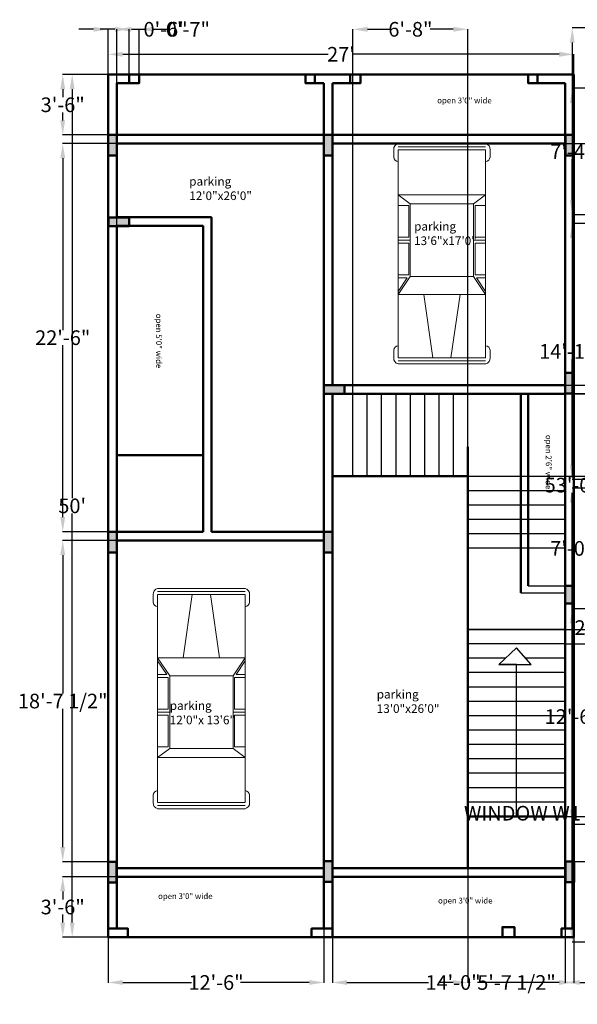
# Model space of a CAD drawing. Units: inches. Extents: x 41 to 5965, y 7 to 3328.
# Tile 1 of 6: x 5054 to 5442, y 1735 to 2420. Entities that reach past the tile are written whole.
import ezdxf

# ---------------------------------------------------------------- set-up
doc = ezdxf.new("R2010")
doc.units = ezdxf.units.IN
doc.header["$MEASUREMENT"] = 0
for name, color, linetype, lineweight in [('A-ANNO-DIMS', 2, 'Continuous', 18), ('A-AREA-IDEN', 3, 'Continuous', 18), ('A-FLOR-STRS', 3, 'Continuous', 25), ('A-FURN', 8, 'Continuous', 18), ('A-WALL', 7, 'Continuous', 50), ('A-WALL-PATT', 8, 'Continuous', 13)]:
    doc.layers.add(name, color=color, linetype=linetype, lineweight=lineweight)
doc.styles.get("Standard").update_dxf_attribs({"font": 'arial.ttf'})
doc.dimstyles.get("Standard").update_dxf_attribs({"dimtxt": 10.18, "dimasz": 10.18, "dimexe": 0.18, "dimexo": 0.0625, "dimgap": 0.09, "dimtad": 0, "dimtih": 1, "dimtoh": 1, "dimdec": 0, "dimzin": 0, "dimdsep": 46, "dimlunit": 3, "dimtxsty": 'Standard', "dimcen": 0.09, "dimadec": 0, "dimazin": 0, "dimtfac": 1, "dimtdec": 0, "dimtofl": 0, "dimtmove": 0, "dimatfit": 3, "dimfxl": 1, "dimtolj": 1, "dimtzin": 0, "dimarcsym": 0})

# ---------------------------------------------------------------- blocks, each defined once
blk = doc.blocks.new('*D1')
at = {"layer": 'A-ANNO-DIMS', "color": 0, "lineweight": -2, "transparency": 16777216}
for p, q in [((5115.3, 2382.15), (5115.3, 2396.38)), ((5125.48, 2396.2), (5268.48, 2396.2)), ((5429.12, 2396.2), (5286.11, 2396.2)), ((5439.3, 2382.15), (5439.3, 2396.38))]:
    blk.add_line(p, q, dxfattribs=at)
at = {"layer": 'A-ANNO-DIMS', "color": 0, "transparency": 16777216}
for points in [[(5125.48, 2397.89), (5125.48, 2394.5), (5115.3, 2396.2)], [(5429.12, 2397.89), (5429.12, 2394.5), (5439.3, 2396.2)]]:
    blk.add_solid(points, dxfattribs=at)
at = {"layer": 'Defpoints', "color": 0, "transparency": 16777216}
for p in [(5439.3, 2396.2), (5115.3, 2382.08), (5439.3, 2382.08)]:
    blk.add_point(p, dxfattribs=at)
at = {"layer": 'A-ANNO-DIMS', "color": 0, "transparency": 16777216, "insert": (5277.3, 2396.2), "char_height": 10.18, "attachment_point": 5}
blk.add_mtext("\\A1;27'", dxfattribs=at)
blk = doc.blocks.new('*D2')
at = {"layer": 'A-ANNO-DIMS', "color": 0, "lineweight": -2, "transparency": 16777216}
for p, q in [((5115.23, 2382.15), (5090.09, 2382.15)), ((5090.27, 2371.97), (5090.27, 2087.4)), ((5090.27, 1792.26), (5090.27, 2076.83)), ((5115.23, 1782.08), (5090.09, 1782.08))]:
    blk.add_line(p, q, dxfattribs=at)
at = {"layer": 'A-ANNO-DIMS', "color": 0, "transparency": 16777216}
for points in [[(5088.57, 2371.97), (5091.96, 2371.97), (5090.27, 2382.15)], [(5088.57, 1792.26), (5091.96, 1792.26), (5090.27, 1782.08)]]:
    blk.add_solid(points, dxfattribs=at)
at = {"layer": 'Defpoints', "color": 0, "transparency": 16777216}
for p in [(5115.3, 2382.15), (5090.27, 1782.08), (5115.3, 1782.08)]:
    blk.add_point(p, dxfattribs=at)
at = {"layer": 'A-ANNO-DIMS', "color": 0, "transparency": 16777216, "insert": (5090.27, 2082.11), "char_height": 10.18, "attachment_point": 5}
blk.add_mtext("\\A1;50'", dxfattribs=at)
blk = doc.blocks.new('*U4')
for p, q in [((0.1, -0.41), (0.1, 38.35)), ((2.77, -0.41), (2.77, 38.31)), ((5.44, 42.31), (12.12, 42.31)), ((5.44, -0.41), (5.44, 38.24)), ((5.45, 38.31), (16.12, 38.31)), ((16.12, 38.31), (180.34, 38.31)), ((61.52, -0.41), (61.52, 38.31)), ((61.52, 38.31), (77.54, 27.62)), ((64.19, 38.31), (76.2, 30.29)), ((76.2, 30.29), (76.2, 38.31)), ((78.87, 38.31), (78.87, 28.96)), ((106.91, 28.96), (106.91, 38.31)), ((109.58, 27.62), (109.58, 38.31)), ((112.25, 38.31), (112.25, 28.96)), ((140.29, 28.96), (140.29, 38.31)), ((141.62, 27.62), (149.64, 38.31)), ((149.64, -0.41), (149.64, 38.31)), ((189.69, 38.31), (179.01, 38.31)), ((189.69, 42.31), (183.01, 42.31)), ((189.69, -0.41), (189.69, 38.24)), ((192.36, -0.41), (192.36, 38.31)), ((195.03, -0.41), (195.03, 38.35)), ((77.54, 27.62), (141.62, 27.62)), ((77.54, -0.41), (77.54, 27.62)), ((78.87, 28.96), (106.91, 28.96)), ((112.25, 28.96), (140.29, 28.96)), ((141.62, -0.41), (141.62, 27.62)), ((5.44, 7.6), (61.52, 15.61)), ((0.1, -0.42), (0.1, -39.18)), ((2.77, -0.41), (2.77, -39.13)), ((5.44, -0.42), (5.44, -39.07)), ((5.44, -8.42), (61.52, -16.43)), ((61.52, -0.41), (61.52, -39.13)), ((77.54, -0.41), (77.54, -28.45)), ((141.62, -0.41), (141.62, -28.45)), ((149.64, -0.41), (149.64, -39.13)), ((189.69, -0.42), (189.69, -39.07)), ((192.36, -0.41), (192.36, -39.13)), ((195.03, -0.42), (195.03, -39.18)), ((61.52, -39.13), (77.54, -28.45)), ((64.19, -39.13), (76.2, -31.12)), ((76.2, -31.12), (76.2, -39.13)), ((77.54, -28.45), (141.62, -28.45)), ((78.87, -39.13), (78.87, -29.79)), ((78.87, -29.79), (106.91, -29.79)), ((106.91, -29.79), (106.91, -39.13)), ((109.58, -28.45), (109.58, -39.13)), ((112.25, -29.79), (140.29, -29.79)), ((112.25, -39.13), (112.25, -29.79)), ((140.29, -29.79), (140.29, -39.13)), ((141.62, -28.45), (149.64, -39.13)), ((5.44, -43.14), (12.12, -43.14)), ((5.45, -39.13), (16.12, -39.13)), ((16.12, -39.13), (180.34, -39.13)), ((189.69, -39.13), (179.01, -39.13)), ((189.69, -43.14), (183.01, -43.14))]:
    blk.add_line(p, q)
for centre, radius, start, end in [((5.06, 37.26), 5.06, 85.64554, 168.0943), ((11.45, 37.64), 4.72, 8.13011, 81.86996), ((183.68, 37.64), 4.72, 98.13004, 171.8699), ((190.07, 37.26), 5.06, 11.90574, 94.35446), ((5.06, -38.09), 5.06, 191.9057, 274.3545), ((11.45, -38.46), 4.72, 278.13, 351.8699), ((183.68, -38.46), 4.72, 188.1301, 261.87), ((190.07, -38.09), 5.06, 265.6455, 348.0943)]:
    blk.add_arc(centre, radius, start, end)
blk = doc.blocks.new('*D20')
at = {"layer": 'A-ANNO-DIMS', "color": 0, "lineweight": -2, "transparency": 16777216}
for p, q in [((5523.49, 1868.32), (5513.31, 1868.32)), ((5523.49, 1860.58), (5523.49, 1868.5)), ((5565.31, 1868.32), (5533.67, 1868.32)), ((5575.49, 1860.58), (5575.49, 1868.5))]:
    blk.add_line(p, q, dxfattribs=at)
at = {"layer": 'A-ANNO-DIMS', "color": 0, "transparency": 16777216}
for points in [[(5533.67, 1870.02), (5533.67, 1866.62), (5523.49, 1868.32)], [(5565.31, 1870.02), (5565.31, 1866.62), (5575.49, 1868.32)]]:
    blk.add_solid(points, dxfattribs=at)
at = {"layer": 'Defpoints', "color": 0, "transparency": 16777216}
for p in [(5523.49, 1868.32), (5523.49, 1860.52), (5575.49, 1860.52)]:
    blk.add_point(p, dxfattribs=at)
at = {"layer": 'A-ANNO-DIMS', "color": 0, "transparency": 16777216, "insert": (5436.17, 1868.32), "char_height": 10.18, "attachment_point": 5}
blk.add_mtext('\\A1;WINDOW W1 4\'-4" TYP.', dxfattribs=at)
blk = doc.blocks.new('*D34')
at = {"layer": 'A-ANNO-DIMS', "color": 0, "lineweight": -2, "transparency": 16777216}
for p, q in [((5105.11, 2413.58), (5094.93, 2413.58)), ((5115.29, 2049.75), (5115.29, 2413.76)), ((5121.29, 2049.75), (5121.29, 2413.76)), ((5131.47, 2413.58), (5141.65, 2413.58))]:
    blk.add_line(p, q, dxfattribs=at)
at = {"layer": 'A-ANNO-DIMS', "color": 0, "transparency": 16777216}
for points in [[(5105.11, 2415.28), (5105.11, 2411.89), (5115.29, 2413.58)], [(5131.47, 2415.28), (5131.47, 2411.89), (5121.29, 2413.58)]]:
    blk.add_solid(points, dxfattribs=at)
at = {"layer": 'Defpoints', "color": 0, "transparency": 16777216}
for p in [(5121.29, 2413.58), (5115.29, 2049.69), (5121.29, 2049.69)]:
    blk.add_point(p, dxfattribs=at)
at = {"layer": 'A-ANNO-DIMS', "color": 0, "transparency": 16777216, "insert": (5155.27, 2413.58), "char_height": 10.18, "attachment_point": 5}
blk.add_mtext('\\A1;0\'-6"', dxfattribs=at)
blk = doc.blocks.new('*D35')
at = {"layer": 'A-ANNO-DIMS', "color": 0, "lineweight": -2, "transparency": 16777216}
for p, q in [((5265.45, 1788.02), (5265.45, 1750.4)), ((5115.3, 1782.02), (5115.3, 1750.4)), ((5125.48, 1750.58), (5173.28, 1750.58)), ((5255.27, 1750.58), (5207.47, 1750.58))]:
    blk.add_line(p, q, dxfattribs=at)
at = {"layer": 'A-ANNO-DIMS', "color": 0, "transparency": 16777216}
for points in [[(5125.48, 1752.28), (5125.48, 1748.89), (5115.3, 1750.58)], [(5255.27, 1752.28), (5255.27, 1748.89), (5265.45, 1750.58)]]:
    blk.add_solid(points, dxfattribs=at)
at = {"layer": 'Defpoints', "color": 0, "transparency": 16777216}
for p in [(5265.45, 1788.08), (5115.3, 1782.08), (5265.45, 1750.58)]:
    blk.add_point(p, dxfattribs=at)
at = {"layer": 'A-ANNO-DIMS', "color": 0, "transparency": 16777216, "insert": (5190.37, 1750.58), "char_height": 10.18, "attachment_point": 5}
blk.add_mtext('\\A1;12\'-6"', dxfattribs=at)
blk = doc.blocks.new('*D36')
at = {"layer": 'A-ANNO-DIMS', "color": 0, "lineweight": -2, "transparency": 16777216}
for p, q in [((5271.3, 1782.02), (5271.3, 1750.4)), ((5439.3, 1782.02), (5439.3, 1750.4)), ((5281.48, 1750.58), (5338.2, 1750.58)), ((5429.12, 1750.58), (5372.39, 1750.58))]:
    blk.add_line(p, q, dxfattribs=at)
at = {"layer": 'A-ANNO-DIMS', "color": 0, "transparency": 16777216}
for points in [[(5281.48, 1752.28), (5281.48, 1748.89), (5271.3, 1750.58)], [(5429.12, 1752.28), (5429.12, 1748.89), (5439.3, 1750.58)]]:
    blk.add_solid(points, dxfattribs=at)
at = {"layer": 'Defpoints', "color": 0, "transparency": 16777216}
for p in [(5271.3, 1782.08), (5439.3, 1782.08), (5439.3, 1750.58)]:
    blk.add_point(p, dxfattribs=at)
at = {"layer": 'A-ANNO-DIMS', "color": 0, "transparency": 16777216, "insert": (5355.3, 1750.58), "char_height": 10.18, "attachment_point": 5}
blk.add_mtext('\\A1;14\'-0"', dxfattribs=at)
blk = doc.blocks.new('*D37')
at = {"layer": 'A-ANNO-DIMS', "color": 0, "lineweight": -2, "transparency": 16777216}
for p, q in [((5121.23, 1824.08), (5083.52, 1824.08)), ((5083.7, 1813.9), (5083.7, 1808.37)), ((5083.7, 1792.26), (5083.7, 1797.79)), ((5115.23, 1782.08), (5083.52, 1782.08))]:
    blk.add_line(p, q, dxfattribs=at)
at = {"layer": 'A-ANNO-DIMS', "color": 0, "transparency": 16777216}
for points in [[(5082, 1813.9), (5085.4, 1813.9), (5083.7, 1824.08)], [(5082, 1792.26), (5085.4, 1792.26), (5083.7, 1782.08)]]:
    blk.add_solid(points, dxfattribs=at)
at = {"layer": 'Defpoints', "color": 0, "transparency": 16777216}
for p in [(5083.7, 1824.08), (5121.3, 1824.08), (5115.3, 1782.08)]:
    blk.add_point(p, dxfattribs=at)
at = {"layer": 'A-ANNO-DIMS', "color": 0, "transparency": 16777216, "insert": (5083.7, 1803.08), "char_height": 10.18, "attachment_point": 5}
blk.add_mtext('\\A1;3\'-6"', dxfattribs=at)
blk = doc.blocks.new('*D38')
at = {"layer": 'A-ANNO-DIMS', "color": 0, "lineweight": -2, "transparency": 16777216}
for p, q in [((5121.23, 2058.08), (5083.52, 2058.08)), ((5083.7, 2047.9), (5083.7, 1951.69)), ((5083.7, 1844.78), (5083.7, 1940.99)), ((5121.14, 1834.6), (5083.52, 1834.6))]:
    blk.add_line(p, q, dxfattribs=at)
at = {"layer": 'A-ANNO-DIMS', "color": 0, "transparency": 16777216}
for points in [[(5082, 2047.9), (5085.4, 2047.9), (5083.7, 2058.08)], [(5082, 1844.78), (5085.4, 1844.78), (5083.7, 1834.6)]]:
    blk.add_solid(points, dxfattribs=at)
at = {"layer": 'Defpoints', "color": 0, "transparency": 16777216}
for p in [(5083.7, 2058.08), (5121.3, 2058.08), (5121.2, 1834.6)]:
    blk.add_point(p, dxfattribs=at)
at = {"layer": 'A-ANNO-DIMS', "color": 0, "transparency": 16777216, "insert": (5083.7, 1946.34), "char_height": 10.18, "attachment_point": 5}
blk.add_mtext('\\A1;18\'-7 1/2"', dxfattribs=at)
blk = doc.blocks.new('*D39')
at = {"layer": 'A-ANNO-DIMS', "color": 0, "lineweight": -2, "transparency": 16777216}
for p, q in [((5121.23, 2334.08), (5083.52, 2334.08)), ((5083.7, 2323.9), (5083.7, 2204.37)), ((5083.7, 2074.26), (5083.7, 2193.79)), ((5121.23, 2064.08), (5083.52, 2064.08))]:
    blk.add_line(p, q, dxfattribs=at)
at = {"layer": 'A-ANNO-DIMS', "color": 0, "transparency": 16777216}
for points in [[(5082, 2323.9), (5085.4, 2323.9), (5083.7, 2334.08)], [(5082, 2074.26), (5085.4, 2074.26), (5083.7, 2064.08)]]:
    blk.add_solid(points, dxfattribs=at)
at = {"layer": 'Defpoints', "color": 0, "transparency": 16777216}
for p in [(5083.7, 2334.08), (5121.3, 2334.08), (5121.3, 2064.08)]:
    blk.add_point(p, dxfattribs=at)
at = {"layer": 'A-ANNO-DIMS', "color": 0, "transparency": 16777216, "insert": (5083.7, 2199.08), "char_height": 10.18, "attachment_point": 5}
blk.add_mtext('\\A1;22\'-6"', dxfattribs=at)
blk = doc.blocks.new('*D40')
at = {"layer": 'A-ANNO-DIMS', "color": 0, "lineweight": -2, "transparency": 16777216}
for p, q in [((5115.23, 2382.08), (5083.52, 2382.08)), ((5083.7, 2371.9), (5083.7, 2366.37)), ((5083.7, 2350.26), (5083.7, 2355.79)), ((5121.23, 2340.08), (5083.52, 2340.08))]:
    blk.add_line(p, q, dxfattribs=at)
at = {"layer": 'A-ANNO-DIMS', "color": 0, "transparency": 16777216}
for points in [[(5082, 2371.9), (5085.4, 2371.9), (5083.7, 2382.08)], [(5082, 2350.26), (5085.4, 2350.26), (5083.7, 2340.08)]]:
    blk.add_solid(points, dxfattribs=at)
at = {"layer": 'Defpoints', "color": 0, "transparency": 16777216}
for p in [(5083.7, 2382.08), (5115.3, 2382.08), (5121.3, 2340.08)]:
    blk.add_point(p, dxfattribs=at)
at = {"layer": 'A-ANNO-DIMS', "color": 0, "transparency": 16777216, "insert": (5083.7, 2361.08), "char_height": 10.18, "attachment_point": 5}
blk.add_mtext('\\A1;3\'-6"', dxfattribs=at)
blk = doc.blocks.new('*D41')
at = {"layer": 'A-ANNO-DIMS', "color": 0, "lineweight": -2, "transparency": 16777216}
for p, q in [((5433.48, 2160.2), (5471.17, 2160.2)), ((5470.99, 2150.02), (5470.99, 2002.77)), ((5470.99, 1844.82), (5470.99, 1992.07)), ((5433.55, 1834.64), (5471.17, 1834.64))]:
    blk.add_line(p, q, dxfattribs=at)
at = {"layer": 'A-ANNO-DIMS', "color": 0, "transparency": 16777216}
for points in [[(5469.29, 2150.02), (5472.69, 2150.02), (5470.99, 2160.2)], [(5469.29, 1844.82), (5472.69, 1844.82), (5470.99, 1834.64)]]:
    blk.add_solid(points, dxfattribs=at)
at = {"layer": 'Defpoints', "color": 0, "transparency": 16777216}
for p in [(5433.42, 2160.2), (5470.99, 2160.2), (5433.49, 1834.64)]:
    blk.add_point(p, dxfattribs=at)
at = {"layer": 'A-ANNO-DIMS', "color": 0, "transparency": 16777216, "insert": (5470.99, 1997.42), "char_height": 10.18, "attachment_point": 5}
blk.add_mtext('\\A1;27\'-1 1/2"', dxfattribs=at)
blk = doc.blocks.new('*D42')
at = {"layer": 'A-ANNO-DIMS', "color": 0, "lineweight": -2, "transparency": 16777216}
for p, q in [((5433.36, 2334.08), (5471.17, 2334.08)), ((5470.99, 2323.9), (5470.99, 2255.37)), ((5470.99, 2176.26), (5470.99, 2244.79)), ((5433.36, 2166.08), (5471.17, 2166.08))]:
    blk.add_line(p, q, dxfattribs=at)
at = {"layer": 'A-ANNO-DIMS', "color": 0, "transparency": 16777216}
for points in [[(5469.29, 2323.9), (5472.69, 2323.9), (5470.99, 2334.08)], [(5469.29, 2176.26), (5472.69, 2176.26), (5470.99, 2166.08)]]:
    blk.add_solid(points, dxfattribs=at)
at = {"layer": 'Defpoints', "color": 0, "transparency": 16777216}
for p in [(5433.3, 2334.08), (5470.99, 2334.08), (5433.3, 2166.08)]:
    blk.add_point(p, dxfattribs=at)
at = {"layer": 'A-ANNO-DIMS', "color": 0, "transparency": 16777216, "insert": (5470.99, 2250.08), "char_height": 10.18, "attachment_point": 5}
blk.add_mtext('\\A1;14\'-0"', dxfattribs=at)
blk = doc.blocks.new('*D43')
at = {"layer": 'A-ANNO-DIMS', "color": 0, "lineweight": -2, "transparency": 16777216}
for p, q in [((5365.62, 1866.02), (5365.62, 1750.4)), ((5433.3, 1866.02), (5433.3, 1750.4)), ((5355.44, 1750.58), (5345.26, 1750.58)), ((5443.48, 1750.58), (5453.66, 1750.58))]:
    blk.add_line(p, q, dxfattribs=at)
at = {"layer": 'A-ANNO-DIMS', "color": 0, "transparency": 16777216}
for points in [[(5355.44, 1752.28), (5355.44, 1748.89), (5365.62, 1750.58)], [(5443.48, 1752.28), (5443.48, 1748.89), (5433.3, 1750.58)]]:
    blk.add_solid(points, dxfattribs=at)
at = {"layer": 'Defpoints', "color": 0, "transparency": 16777216}
for p in [(5365.62, 1866.08), (5433.3, 1866.08), (5433.3, 1750.58)]:
    blk.add_point(p, dxfattribs=at)
at = {"layer": 'A-ANNO-DIMS', "color": 0, "transparency": 16777216, "insert": (5399.46, 1750.58), "char_height": 10.18, "attachment_point": 5}
blk.add_mtext('\\A1;5\'-7 1/2"', dxfattribs=at)
blk = doc.blocks.new('*D44')
at = {"layer": 'A-ANNO-DIMS', "color": 0, "lineweight": -2, "transparency": 16777216}
for p, q in [((5470.99, 2006.26), (5470.99, 2016.44)), ((5470.99, 2016.44), (5481.17, 2016.44)), ((5433.36, 1996.08), (5471.17, 1996.08)), ((5433.36, 1986.08), (5471.17, 1986.08)), ((5470.99, 1975.9), (5470.99, 1965.72))]:
    blk.add_line(p, q, dxfattribs=at)
at = {"layer": 'A-ANNO-DIMS', "color": 0, "transparency": 16777216}
for points in [[(5469.29, 2006.26), (5472.69, 2006.26), (5470.99, 1996.08)], [(5469.29, 1975.9), (5472.69, 1975.9), (5470.99, 1986.08)]]:
    blk.add_solid(points, dxfattribs=at)
at = {"layer": 'Defpoints', "color": 0, "transparency": 16777216}
for p in [(5433.3, 1996.08), (5470.99, 1996.08), (5433.3, 1986.08)]:
    blk.add_point(p, dxfattribs=at)
at = {"layer": 'A-ANNO-DIMS', "color": 0, "transparency": 16777216, "insert": (5498.75, 2016.44), "char_height": 10.18, "attachment_point": 5}
blk.add_mtext('\\A1;0\'-10"', dxfattribs=at)
blk = doc.blocks.new('*D45')
at = {"layer": 'A-ANNO-DIMS', "color": 0, "lineweight": -2, "transparency": 16777216}
for p, q in [((5365.69, 1996.08), (5471.17, 1996.08)), ((5470.99, 1985.9), (5470.99, 1936.37)), ((5470.99, 1876.26), (5470.99, 1925.79)), ((5365.69, 1866.08), (5471.17, 1866.08))]:
    blk.add_line(p, q, dxfattribs=at)
at = {"layer": 'A-ANNO-DIMS', "color": 0, "transparency": 16777216}
for points in [[(5469.29, 1985.9), (5472.69, 1985.9), (5470.99, 1996.08)], [(5469.29, 1876.26), (5472.69, 1876.26), (5470.99, 1866.08)]]:
    blk.add_solid(points, dxfattribs=at)
at = {"layer": 'Defpoints', "color": 0, "transparency": 16777216}
for p in [(5365.62, 1996.08), (5470.99, 1996.08), (5365.62, 1866.08)]:
    blk.add_point(p, dxfattribs=at)
at = {"layer": 'A-ANNO-DIMS', "color": 0, "transparency": 16777216, "insert": (5470.99, 1931.08), "char_height": 10.18, "attachment_point": 5}
blk.add_mtext('\\A1;10\'-10"', dxfattribs=at)
blk = doc.blocks.new('*D46')
at = {"layer": 'A-ANNO-DIMS', "color": 0, "lineweight": -2, "transparency": 16777216}
for p, q in [((5365.69, 2160.08), (5471.17, 2160.08)), ((5470.99, 2149.9), (5470.99, 2136.75)), ((5470.99, 2113.02), (5470.99, 2126.17)), ((5365.69, 2102.84), (5471.17, 2102.84))]:
    blk.add_line(p, q, dxfattribs=at)
at = {"layer": 'A-ANNO-DIMS', "color": 0, "transparency": 16777216}
for points in [[(5469.29, 2149.9), (5472.69, 2149.9), (5470.99, 2160.08)], [(5469.29, 2113.02), (5472.69, 2113.02), (5470.99, 2102.84)]]:
    blk.add_solid(points, dxfattribs=at)
at = {"layer": 'Defpoints', "color": 0, "transparency": 16777216}
for p in [(5365.62, 2160.08), (5470.99, 2160.08), (5365.62, 2102.84)]:
    blk.add_point(p, dxfattribs=at)
at = {"layer": 'A-ANNO-DIMS', "color": 0, "transparency": 16777216, "insert": (5470.99, 2131.46), "char_height": 10.18, "attachment_point": 5}
blk.add_mtext('\\A1;4\'-9"', dxfattribs=at)
blk = doc.blocks.new('*D47')
at = {"layer": 'A-ANNO-DIMS', "color": 0, "lineweight": -2, "transparency": 16777216}
for p, q in [((5285.62, 2102.9), (5285.62, 2413.76)), ((5295.8, 2413.58), (5311.97, 2413.58)), ((5355.44, 2413.58), (5339.27, 2413.58)), ((5365.62, 2102.9), (5365.62, 2413.76))]:
    blk.add_line(p, q, dxfattribs=at)
at = {"layer": 'A-ANNO-DIMS', "color": 0, "transparency": 16777216}
for points in [[(5295.8, 2415.28), (5295.8, 2411.89), (5285.62, 2413.58)], [(5355.44, 2415.28), (5355.44, 2411.89), (5365.62, 2413.58)]]:
    blk.add_solid(points, dxfattribs=at)
at = {"layer": 'Defpoints', "color": 0, "transparency": 16777216}
for p in [(5365.62, 2413.58), (5285.62, 2102.84), (5365.62, 2102.84)]:
    blk.add_point(p, dxfattribs=at)
at = {"layer": 'A-ANNO-DIMS', "color": 0, "transparency": 16777216, "insert": (5325.62, 2413.58), "char_height": 10.18, "attachment_point": 5}
blk.add_mtext('\\A1;6\'-8"', dxfattribs=at)
blk = doc.blocks.new('*D48')
at = {"layer": 'A-ANNO-DIMS', "color": 0, "lineweight": -2, "transparency": 16777216}
for p, q in [((5119.86, 2413.58), (5109.68, 2413.58)), ((5130.04, 2382.15), (5130.04, 2413.76)), ((5136.83, 2376.15), (5136.83, 2413.76)), ((5147.01, 2413.58), (5157.19, 2413.58))]:
    blk.add_line(p, q, dxfattribs=at)
at = {"layer": 'A-ANNO-DIMS', "color": 0, "transparency": 16777216}
for points in [[(5119.86, 2415.28), (5119.86, 2411.89), (5130.04, 2413.58)], [(5147.01, 2415.28), (5147.01, 2411.89), (5136.83, 2413.58)]]:
    blk.add_solid(points, dxfattribs=at)
at = {"layer": 'Defpoints', "color": 0, "transparency": 16777216}
for p in [(5136.83, 2413.58), (5130.04, 2382.08), (5136.83, 2376.08)]:
    blk.add_point(p, dxfattribs=at)
at = {"layer": 'A-ANNO-DIMS', "color": 0, "transparency": 16777216, "insert": (5170.81, 2413.58), "char_height": 10.18, "attachment_point": 5}
blk.add_mtext('\\A1;0\'-7"', dxfattribs=at)
blk = doc.blocks.new('*D50')
at = {"layer": 'A-ANNO-DIMS', "color": 0, "lineweight": -2, "transparency": 16777216}
for p, q in [((5471.43, 2414.52), (5438.06, 2414.52)), ((5438.24, 2404.34), (5438.24, 2101.81)), ((5438.24, 1788.7), (5438.24, 2091.23)), ((5471.43, 1778.52), (5438.06, 1778.52))]:
    blk.add_line(p, q, dxfattribs=at)
at = {"layer": 'A-ANNO-DIMS', "color": 0, "transparency": 16777216}
for points in [[(5436.55, 2404.34), (5439.94, 2404.34), (5438.24, 2414.52)], [(5436.55, 1788.7), (5439.94, 1788.7), (5438.24, 1778.52)]]:
    blk.add_solid(points, dxfattribs=at)
at = {"layer": 'Defpoints', "color": 0, "transparency": 16777216}
for p in [(5438.24, 2414.52), (5471.49, 2414.52), (5471.49, 1778.52)]:
    blk.add_point(p, dxfattribs=at)
at = {"layer": 'A-ANNO-DIMS', "color": 0, "transparency": 16777216, "insert": (5438.24, 2096.52), "char_height": 10.18, "attachment_point": 5}
blk.add_mtext('\\A1;53\'-0"', dxfattribs=at)
blk = doc.blocks.new('*D59')
at = {"layer": 'A-ANNO-DIMS', "color": 0, "lineweight": -2, "transparency": 16777216}
for p, q in [((5477.43, 2010.52), (5438.06, 2010.52)), ((5438.24, 2000.34), (5438.24, 1940.81)), ((5438.24, 1870.7), (5438.24, 1930.23)), ((5477.43, 1860.52), (5438.06, 1860.52))]:
    blk.add_line(p, q, dxfattribs=at)
at = {"layer": 'A-ANNO-DIMS', "color": 0, "transparency": 16777216}
for points in [[(5436.55, 2000.34), (5439.94, 2000.34), (5438.24, 2010.52)], [(5436.55, 1870.7), (5439.94, 1870.7), (5438.24, 1860.52)]]:
    blk.add_solid(points, dxfattribs=at)
at = {"layer": 'Defpoints', "color": 0, "transparency": 16777216}
for p in [(5438.24, 2010.52), (5477.49, 2010.52), (5477.49, 1860.52)]:
    blk.add_point(p, dxfattribs=at)
at = {"layer": 'A-ANNO-DIMS', "color": 0, "transparency": 16777216, "insert": (5438.24, 1935.52), "char_height": 10.18, "attachment_point": 5}
blk.add_mtext('\\A1;12\'-6"', dxfattribs=at)
blk = doc.blocks.new('*D60')
at = {"layer": 'A-ANNO-DIMS', "color": 0, "lineweight": -2, "transparency": 16777216}
for p, q in [((5477.43, 2094.52), (5438.06, 2094.52)), ((5438.24, 2084.34), (5438.24, 2057.81)), ((5438.24, 2020.7), (5438.24, 2047.23)), ((5477.43, 2010.52), (5438.06, 2010.52))]:
    blk.add_line(p, q, dxfattribs=at)
at = {"layer": 'A-ANNO-DIMS', "color": 0, "transparency": 16777216}
for points in [[(5436.55, 2084.34), (5439.94, 2084.34), (5438.24, 2094.52)], [(5436.55, 2020.7), (5439.94, 2020.7), (5438.24, 2010.52)]]:
    blk.add_solid(points, dxfattribs=at)
at = {"layer": 'Defpoints', "color": 0, "transparency": 16777216}
for p in [(5438.24, 2094.52), (5477.49, 2094.52), (5477.49, 2010.52)]:
    blk.add_point(p, dxfattribs=at)
at = {"layer": 'A-ANNO-DIMS', "color": 0, "transparency": 16777216, "insert": (5438.24, 2052.52), "char_height": 10.18, "attachment_point": 5}
blk.add_mtext('\\A1;7\'-0"', dxfattribs=at)
blk = doc.blocks.new('*D61')
at = {"layer": 'A-ANNO-DIMS', "color": 0, "lineweight": -2, "transparency": 16777216}
for p, q in [((5477.43, 2278.52), (5438.06, 2278.52)), ((5438.24, 2268.34), (5438.24, 2194.81)), ((5438.24, 2110.7), (5438.24, 2184.23)), ((5477.43, 2100.52), (5438.06, 2100.52))]:
    blk.add_line(p, q, dxfattribs=at)
at = {"layer": 'A-ANNO-DIMS', "color": 0, "transparency": 16777216}
for points in [[(5436.55, 2268.34), (5439.94, 2268.34), (5438.24, 2278.52)], [(5436.55, 2110.7), (5439.94, 2110.7), (5438.24, 2100.52)]]:
    blk.add_solid(points, dxfattribs=at)
at = {"layer": 'Defpoints', "color": 0, "transparency": 16777216}
for p in [(5438.24, 2278.52), (5477.49, 2278.52), (5477.49, 2100.52)]:
    blk.add_point(p, dxfattribs=at)
at = {"layer": 'A-ANNO-DIMS', "color": 0, "transparency": 16777216, "insert": (5438.24, 2189.52), "char_height": 10.18, "attachment_point": 5}
blk.add_mtext('\\A1;14\'-10"', dxfattribs=at)
blk = doc.blocks.new('*D62')
at = {"layer": 'A-ANNO-DIMS', "color": 0, "lineweight": -2, "transparency": 16777216}
for p, q in [((5477.43, 2372.52), (5438.06, 2372.52)), ((5438.24, 2362.34), (5438.24, 2333.7)), ((5438.24, 2294.7), (5438.24, 2323.34)), ((5477.43, 2284.52), (5438.06, 2284.52))]:
    blk.add_line(p, q, dxfattribs=at)
at = {"layer": 'A-ANNO-DIMS', "color": 0, "transparency": 16777216}
for points in [[(5436.55, 2362.34), (5439.94, 2362.34), (5438.24, 2372.52)], [(5436.55, 2294.7), (5439.94, 2294.7), (5438.24, 2284.52)]]:
    blk.add_solid(points, dxfattribs=at)
at = {"layer": 'Defpoints', "color": 0, "transparency": 16777216}
for p in [(5438.24, 2372.52), (5477.49, 2372.52), (5477.49, 2284.52)]:
    blk.add_point(p, dxfattribs=at)
at = {"layer": 'A-ANNO-DIMS', "color": 0, "transparency": 16777216, "insert": (5438.24, 2328.52), "char_height": 10.18, "attachment_point": 5}
blk.add_mtext('\\A1;7\'-4"', dxfattribs=at)

msp = doc.modelspace()

# ---------------------------------------------------------------- hatches: boundary and pattern name
at = {"layer": 'A-WALL-PATT'}
h = msp.add_hatch(color=256, dxfattribs=at)
h.dxf.hatch_style = 1
h.paths.add_polyline_path([(5121.29, 2064.05), (5115.3, 2064.05), (5115.3, 2049.69), (5121.29, 2049.69)])
h.paths.add_polyline_path([(5271.3, 2064.12), (5265.49, 2064.12), (5265.49, 2049.75), (5271.3, 2049.75)])
h.paths.add_polyline_path([(5121.2, 1834.6), (5115.3, 1834.6), (5115.3, 1820.23), (5121.2, 1820.23)])
h.paths.add_polyline_path([(5271.3, 1834.94), (5265.48, 1834.94), (5265.48, 1820.58), (5271.3, 1820.58)])
h.paths.add_polyline_path([(5439.3, 1834.64), (5433.49, 1834.64), (5433.49, 1820.28), (5439.3, 1820.28)])
h.paths.add_polyline_path([(5439.3, 2340.08), (5433.45, 2340.08), (5433.45, 2325.72), (5439.3, 2325.72)])
h.paths.add_polyline_path([(5271.3, 2340.08), (5265.39, 2340.08), (5265.39, 2325.72), (5271.3, 2325.72)])
h.paths.add_polyline_path([(5121.3, 2340.08), (5115.3, 2340.08), (5115.3, 2325.72), (5121.3, 2325.72)])
h.paths.add_polyline_path([(5439.3, 2174.56), (5433.42, 2174.56), (5433.42, 2160.2), (5439.3, 2160.2)])
h = msp.add_hatch(color=256, dxfattribs=at)
h.dxf.hatch_style = 1
h.paths.add_polyline_path([(5129.99, 2282.69), (5115.62, 2282.69), (5115.62, 2276.69), (5121.54, 2276.69), (5121.54, 2276.84), (5129.99, 2276.84)])
h = msp.add_hatch(color=256, dxfattribs=at)
h.dxf.hatch_style = 1
h.paths.add_polyline_path([(5279.74, 2165.94), (5265.38, 2165.94), (5265.38, 2159.94), (5271.3, 2159.94), (5271.3, 2160.08), (5279.74, 2160.08)])
h = msp.add_hatch(color=256, dxfattribs=at)
h.dxf.hatch_style = 1
h.paths.add_polyline_path([(5433.3, 2014.29), (5439.3, 2014.29), (5439.3, 2026.39), (5433.3, 2026.39)])

# ---------------------------------------------------------------- linework, layer by layer
at = {"layer": 'A-FLOR-STRS'}
for p, q in [((5285.62, 2123.14), (5285.62, 2160.08)), ((5295.62, 2123.14), (5295.62, 2160.08)), ((5305.62, 2123.14), (5305.62, 2160.08)), ((5315.62, 2123.14), (5315.62, 2160.08)), ((5325.62, 2123.14), (5325.62, 2160.08)), ((5335.62, 2123.14), (5335.62, 2160.08)), ((5345.62, 2123.14), (5345.62, 2160.08)), ((5355.62, 2123.14), (5355.62, 2160.08)), ((5365.62, 2123.14), (5365.62, 2160.08)), ((5285.62, 2102.84), (5285.62, 2123.14)), ((5295.62, 2102.84), (5295.62, 2123.14)), ((5305.62, 2102.84), (5305.62, 2123.14)), ((5315.62, 2102.84), (5315.62, 2123.14)), ((5325.62, 2102.84), (5325.62, 2123.14)), ((5335.62, 2102.84), (5335.62, 2123.14)), ((5345.62, 2102.84), (5345.62, 2123.14)), ((5355.62, 2102.84), (5355.62, 2123.14)), ((5365.62, 2102.84), (5433.3, 2102.84)), ((5365.62, 2092.84), (5433.3, 2092.84)), ((5365.62, 2082.84), (5433.3, 2082.84)), ((5365.62, 2072.84), (5433.3, 2072.84)), ((5365.62, 2062.84), (5433.3, 2062.84)), ((5365.62, 2052.84), (5433.3, 2052.84)), ((5402.49, 2021.56), (5433.3, 2021.56)), ((5407.52, 2026.39), (5433.3, 2026.39)), ((5433.3, 1996.08), (5365.62, 1996.08)), ((5433.3, 1986.08), (5365.62, 1986.08)), ((5399.46, 1983.24), (5387.09, 1971.84)), ((5409.56, 1971.84), (5399.46, 1983.24)), ((5391.69, 1976.08), (5365.62, 1976.08)), ((5433.3, 1976.08), (5405.8, 1976.08)), ((5433.3, 1966.08), (5365.62, 1966.08)), ((5399.46, 1971.84), (5387.09, 1971.84)), ((5387.09, 1971.84), (5409.56, 1971.84)), ((5399.46, 1866.08), (5399.46, 1971.84)), ((5433.3, 1956.08), (5365.62, 1956.08)), ((5433.3, 1946.08), (5365.62, 1946.08)), ((5433.3, 1936.08), (5365.62, 1936.08)), ((5433.3, 1926.08), (5365.62, 1926.08)), ((5433.3, 1916.08), (5365.62, 1916.08)), ((5433.3, 1906.08), (5365.62, 1906.08)), ((5433.3, 1896.08), (5365.62, 1896.08)), ((5433.3, 1886.08), (5365.62, 1886.08)), ((5433.3, 1876.08), (5365.62, 1876.08))]:
    msp.add_line(p, q, dxfattribs=at)
at = {"layer": 'A-WALL'}
for p, q in [((5115.3, 1782.08), (5115.3, 2382.08)), ((5115.3, 2382.08), (5439.3, 2382.08)), ((5439.3, 2382.08), (5439.3, 1782.08)), ((5121.3, 2376.08), (5136.83, 2376.08)), ((5121.3, 2282.82), (5121.3, 2376.08)), ((5252.65, 2376.08), (5265.3, 2376.08)), ((5265.3, 1788.08), (5265.3, 2376.08)), ((5271.3, 2166.08), (5271.3, 2376.08)), ((5271.3, 2376.08), (5290.87, 2376.08)), ((5407.67, 2376.08), (5433.3, 2376.08)), ((5433.3, 2376.08), (5433.3, 1788.08)), ((5121.3, 2340.08), (5433.3, 2340.08)), ((5121.3, 2334.08), (5181.3, 2334.08)), ((5121.3, 2334.08), (5265.39, 2334.08)), ((5271.3, 2334.08), (5433.3, 2334.08)), ((5181.3, 2282.82), (5121.3, 2282.82)), ((5181.3, 2282.82), (5187.3, 2282.82)), ((5187.3, 2064.08), (5187.3, 2282.82)), ((5121.3, 1788.08), (5121.3, 2276.82)), ((5181.3, 2276.82), (5121.3, 2276.82)), ((5181.3, 2064.08), (5181.3, 2276.82)), ((5271.3, 2166.08), (5433.3, 2166.08)), ((5271.3, 2160.08), (5433.3, 2160.08)), ((5271.3, 1788.08), (5271.3, 2160.08)), ((5402.49, 2160.08), (5402.49, 2021.56)), ((5407.52, 2160.08), (5407.52, 2026.39)), ((5365.62, 1830.08), (5365.62, 2123.14)), ((5181.3, 2117.35), (5121.3, 2117.35)), ((5365.62, 2102.84), (5271.3, 2102.84)), ((5121.3, 2064.08), (5181.3, 2064.08)), ((5187.3, 2064.08), (5265.3, 2064.08)), ((5121.3, 2058.08), (5265.47, 2058.08)), ((5433.3, 1866.08), (5365.62, 1866.08)), ((5265.45, 1830.08), (5121.3, 1830.08)), ((5433.3, 1830.08), (5271.3, 1830.08)), ((5265.45, 1824.08), (5121.3, 1824.08)), ((5433.3, 1824.08), (5271.3, 1824.08)), ((5129.06, 1788.08), (5121.3, 1788.08)), ((5265.45, 1788.08), (5256.82, 1788.08)), ((5433.3, 1788.08), (5430.7, 1788.08)), ((5439.3, 1782.08), (5115.3, 1782.08))]:
    msp.add_line(p, q, dxfattribs=at)
for points in [[(5130.04, 2376.08), (5136.83, 2376.08), (5136.83, 2382.08), (5130.04, 2382.08)], [(5259.07, 2376.08), (5252.65, 2376.08), (5252.65, 2382.08), (5259.07, 2382.08)], [(5283.75, 2376.08), (5290.87, 2376.08), (5290.87, 2382.08), (5283.75, 2382.08)], [(5414.11, 2376.08), (5407.67, 2376.08), (5407.67, 2382.08), (5414.11, 2382.08)], [(5121.3, 2340.08), (5115.3, 2340.08), (5115.3, 2325.72), (5121.3, 2325.72)], [(5271.39, 2340.08), (5265.39, 2340.08), (5265.39, 2325.72), (5271.39, 2325.72)], [(5439.45, 2340.08), (5433.45, 2340.08), (5433.45, 2325.72), (5439.45, 2325.72)], [(5129.99, 2276.69), (5129.99, 2282.69), (5115.62, 2282.69), (5115.62, 2276.69)], [(5129.99, 2276.69), (5129.99, 2282.69), (5115.62, 2282.69), (5115.62, 2276.69)], [(5439.42, 2174.56), (5433.42, 2174.56), (5433.42, 2160.2), (5439.42, 2160.2)], [(5279.74, 2159.94), (5279.74, 2165.94), (5265.38, 2165.94), (5265.38, 2159.94)], [(5279.74, 2159.94), (5279.74, 2165.94), (5265.38, 2165.94), (5265.38, 2159.94)], [(5121.29, 2064.05), (5115.29, 2064.05), (5115.29, 2049.69), (5121.29, 2049.69)], [(5271.49, 2064.12), (5265.49, 2064.12), (5265.49, 2049.75), (5271.49, 2049.75)], [(5433.3, 2026.39), (5439.3, 2026.39), (5439.3, 2014.29), (5433.3, 2014.29)], [(5121.2, 1834.6), (5115.2, 1834.6), (5115.2, 1820.23), (5121.2, 1820.23)], [(5271.48, 1834.94), (5265.48, 1834.94), (5265.48, 1820.58), (5271.48, 1820.58)], [(5439.49, 1834.64), (5433.49, 1834.64), (5433.49, 1820.28), (5439.49, 1820.28)], [(5115.3, 1788.08), (5129.06, 1788.08), (5129.06, 1782.08), (5115.3, 1782.08)], [(5271.3, 1788.08), (5256.82, 1788.08), (5256.82, 1782.08), (5271.3, 1782.08)], [(5389.65, 1782.08), (5397.98, 1782.08), (5397.98, 1789.17), (5389.65, 1789.17)], [(5439.3, 1782.08), (5430.7, 1782.08), (5430.7, 1788.08), (5439.3, 1788.08)]]:
    msp.add_lwpolyline(points, close=True, dxfattribs=at)

# ---------------------------------------------------------------- block references
at = {"layer": 'A-FURN', "xscale": 0.7856366796747984, "yscale": 0.7856366796747984, "zscale": 0.7856366796747984}
for p, rotation in [((5347.24, 2180.81), 90), ((5180.48, 2024.7), 270)]:
    msp.add_blockref('*U4', p, dxfattribs=dict(at, rotation=rotation))

# ---------------------------------------------------------------- texts
at = {"layer": 'A-AREA-IDEN', "attachment_point": 1}
for s, width, insert, char_height in [('open 3\'0" wide', 93.5361, (5344.28, 2366.06), 4), ('parking\\P12\'0"x26\'0"', 93.5984, (5171.7, 2310.81), 6), ('parking\\P13\'6"x17\'0"', 93.5984, (5328.18, 2279.52), 6), ('parking\\P13\'0"x26\'0"', 93.5984, (5302.18, 1954.07), 6), ('parking\\P12\'0"x 13\'6"', 93.5984, (5158.13, 1946.18), 6), ('open 3\'0" wide', 93.5361, (5150.04, 1812.62), 4), ('open 3\'0" wide', 93.5361, (5344.84, 1809.53), 4)]:
    msp.add_mtext_dynamic_manual_height_columns(s, width=width, gutter_width=1, heights=[0], dxfattribs=dict(at, insert=insert, char_height=char_height))
at = {"layer": 'A-AREA-IDEN', "char_height": 4, "attachment_point": 1, "rotation": 270}
for s, insert in [('open 5\'0" wide', (5152.62, 2215.7)), ('open 2\'6" wide', (5423.83, 2131.48))]:
    msp.add_mtext_dynamic_manual_height_columns(s, width=93.5361, gutter_width=1, heights=[0], dxfattribs=dict(at, insert=insert))

# ---------------------------------------------------------------- dimensions: what is measured, and where the dimension line sits
at = {"layer": 'A-ANNO-DIMS'}
for base, p1, p2, override, picture, middle in [((5121.29, 2413.58), (5115.29, 2049.69), (5121.29, 2049.69), {"dimdec": 1, "dimlfac": 1, "dimrnd": 0, "dimzin": 1, "dimdsep": 46, "dimlunit": 4, "dimfrac": 2}, '*D34', (5155.27, 2413.58)), ((5136.83, 2413.58), (5130.04, 2382.08), (5136.83, 2376.08), {"dimdec": 1, "dimlfac": 1, "dimrnd": 0, "dimzin": 1, "dimdsep": 46, "dimlunit": 4, "dimfrac": 2}, '*D48', (5170.81, 2413.58)), ((5365.62, 2413.58), (5285.62, 2102.84), (5365.62, 2102.84), {"dimdec": 1, "dimlfac": 1, "dimrnd": 0, "dimzin": 1, "dimdsep": 46, "dimlunit": 4, "dimfrac": 2}, '*D47', (5325.62, 2413.58)), ((5439.3, 2396.2), (5115.3, 2382.08), (5439.3, 2382.08), {"dimclrd": 0, "dimclre": 0, "dimclrt": 0}, '*D1', (5277.3, 2396.2)), ((5433.3, 1750.58), (5365.62, 1866.08), (5433.3, 1866.08), {"dimdec": 1, "dimlfac": 1, "dimrnd": 0, "dimzin": 1, "dimdsep": 46, "dimlunit": 4, "dimfrac": 2}, '*D43', (5399.46, 1750.58)), ((5265.4458, 1750.5826), (5115.297, 1782.0826), (5265.4458, 1788.0826), {"dimdec": 1, "dimlfac": 1, "dimrnd": 0, "dimzin": 1, "dimdsep": 46, "dimlunit": 4, "dimfrac": 2}, '*D35', (5190.3714, 1750.5826)), ((5439.3, 1750.58), (5271.3, 1782.08), (5439.3, 1782.08), {"dimdec": 1, "dimlfac": 1, "dimrnd": 0, "dimzin": 1, "dimdsep": 46, "dimlunit": 4, "dimfrac": 2}, '*D36', (5355.3, 1750.58))]:
    dim = msp.add_linear_dim(base=base, p1=p1, p2=p2, dimstyle='Standard', override=override, dxfattribs=at)
    dim.commit()
    dim.dimension.update_dxf_attribs({"geometry": picture, "text_midpoint": middle})
for base, p1, p2, override, picture, middle in [((5438.24, 2414.52), (5471.49, 1778.52), (5471.49, 2414.52), {"dimdec": 1, "dimlfac": 1, "dimrnd": 0, "dimzin": 1, "dimdsep": 46, "dimlunit": 4, "dimfrac": 2}, '*D50', (5438.24, 2096.52)), ((5083.7, 2382.08), (5121.3, 2340.08), (5115.3, 2382.08), {"dimdec": 1, "dimlfac": 1, "dimrnd": 0, "dimzin": 1, "dimdsep": 46, "dimlunit": 4, "dimfrac": 2}, '*D40', (5083.7, 2361.08)), ((5090.27, 1782.08), (5115.3, 2382.15), (5115.3, 1782.08), {"dimclrd": 0, "dimclre": 0, "dimclrt": 0}, '*D2', (5090.27, 2082.11)), ((5438.24, 2372.52), (5477.49, 2284.52), (5477.49, 2372.52), {"dimdec": 1, "dimlfac": 1, "dimrnd": 0, "dimzin": 1, "dimdsep": 46, "dimlunit": 4, "dimfrac": 2}, '*D62', (5438.24, 2328.52)), ((5083.7, 2334.08), (5121.3, 2064.08), (5121.3, 2334.08), {"dimdec": 1, "dimlfac": 1, "dimrnd": 0, "dimzin": 1, "dimdsep": 46, "dimlunit": 4, "dimfrac": 2}, '*D39', (5083.7, 2199.08)), ((5470.99, 2334.08), (5433.3, 2166.08), (5433.3, 2334.08), {"dimdec": 1, "dimlfac": 1, "dimrnd": 0, "dimzin": 1, "dimdsep": 46, "dimlunit": 4, "dimfrac": 2}, '*D42', (5470.99, 2250.08)), ((5438.24, 2278.52), (5477.49, 2100.52), (5477.49, 2278.52), {"dimdec": 1, "dimlfac": 1, "dimrnd": 0, "dimzin": 1, "dimdsep": 46, "dimlunit": 4, "dimfrac": 2}, '*D61', (5438.24, 2189.52)), ((5470.99, 2160.08), (5365.62, 2102.84), (5365.62, 2160.08), {"dimdec": 1, "dimlfac": 1, "dimrnd": 0, "dimzin": 1, "dimdsep": 46, "dimlunit": 4, "dimfrac": 2}, '*D46', (5470.99, 2131.46)), ((5470.99, 2160.2), (5433.49, 1834.64), (5433.42, 2160.2), {"dimdec": 1, "dimlfac": 1, "dimrnd": 0, "dimzin": 1, "dimdsep": 46, "dimlunit": 4, "dimfrac": 2}, '*D41', (5470.99, 1997.42)), ((5438.24, 2094.52), (5477.49, 2010.52), (5477.49, 2094.52), {"dimdec": 1, "dimlfac": 1, "dimrnd": 0, "dimzin": 1, "dimdsep": 46, "dimlunit": 4, "dimfrac": 2}, '*D60', (5438.24, 2052.52)), ((5083.7, 2058.08), (5121.2, 1834.6), (5121.3, 2058.08), {"dimdec": 1, "dimlfac": 1, "dimrnd": 0, "dimzin": 1, "dimdsep": 46, "dimlunit": 4, "dimfrac": 2}, '*D38', (5083.7, 1946.34)), ((5470.99, 1996.08), (5433.3, 1986.08), (5433.3, 1996.08), {"dimdec": 1, "dimlfac": 1, "dimrnd": 0, "dimzin": 1, "dimdsep": 46, "dimlunit": 4, "dimfrac": 2}, '*D44', (5498.75, 2016.44)), ((5438.24, 2010.52), (5477.49, 1860.52), (5477.49, 2010.52), {"dimdec": 1, "dimlfac": 1, "dimrnd": 0, "dimzin": 1, "dimdsep": 46, "dimlunit": 4, "dimfrac": 2}, '*D59', (5438.24, 1935.52)), ((5470.99, 1996.08), (5365.62, 1866.08), (5365.62, 1996.08), {"dimdec": 1, "dimlfac": 1, "dimrnd": 0, "dimzin": 1, "dimdsep": 46, "dimlunit": 4, "dimfrac": 2}, '*D45', (5470.99, 1931.08)), ((5083.7, 1824.08), (5115.3, 1782.08), (5121.3, 1824.08), {"dimdec": 1, "dimlfac": 1, "dimrnd": 0, "dimzin": 1, "dimdsep": 46, "dimlunit": 4, "dimfrac": 2}, '*D37', (5083.7, 1803.08))]:
    dim = msp.add_linear_dim(base=base, p1=p1, p2=p2, angle=90, dimstyle='Standard', override=override, dxfattribs=at)
    dim.commit()
    dim.dimension.update_dxf_attribs({"geometry": picture, "text_midpoint": middle})
dim = msp.add_linear_dim(base=(5523.49, 1868.32), p1=(5575.49, 1860.52), p2=(5523.49, 1860.52), angle=180, text='WINDOW W1 <> TYP.', dimstyle='Standard', override={"dimdec": 1, "dimrnd": 0, "dimzin": 1, "dimlunit": 4, "dimfrac": 2}, dxfattribs=at)
dim.commit()
dim.dimension.update_dxf_attribs({"geometry": '*D20', "text_midpoint": (5436.17, 1868.32)})

doc.saveas('drawing.dxf')
